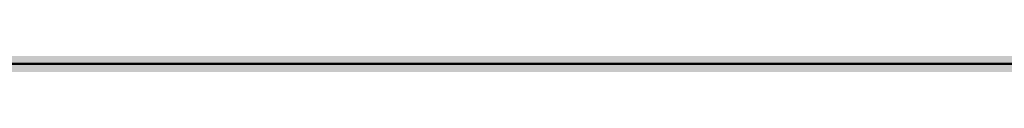
# Model space of a CAD drawing. Units: millimetres. Extents: x 0 to 2267, y 0 to 1823.
# Tile 113 of 256: x 1600.369 to 1605.705, y 1232.247 to 1232.247. Entities that reach past the tile are written whole.
import ezdxf

# ---------------------------------------------------------------- set-up
doc = ezdxf.new("R2010")
doc.units = ezdxf.units.MM
doc.header["$MEASUREMENT"] = 0
doc.layers.add('M-HATC', color=252, linetype='Continuous', lineweight=18)
doc.layers.add('M-OUTL', color=7, linetype='Continuous', lineweight=50)

msp = doc.modelspace()

# ---------------------------------------------------------------- hatches: boundary and pattern name
at = {"layer": 'M-HATC'}
h = msp.add_hatch(color=256, dxfattribs=at)
h.dxf.hatch_style = 1
h.paths.add_polyline_path([(2065.771, 1618.062, 0.236068), (2055.771, 1638.062), (1381.0868, 1638.062, 0.236068), (1371.0868, 1618.062), (1371.0868, 1603.062), (2055.771, 1603.062), (2065.771, 1603.062)])
h.paths.add_polyline_path([(2062.7718, 1550.2964), (2062.7718, 1560.2964), (1374.086, 1560.2964), (1374.086, 1550.2964), (1374.086, 1540.2964), (1384.086, 1540.2964), (1389.086, 1540.2964), (2062.7718, 1540.2964)])
h.paths.add_polyline_path([(1930.9289, 1282.7656), (1505.9289, 1282.7656), (1587.6276, 1235.5968, 0.131652), (1600.1276, 1232.2475), (1836.7302, 1232.2475, 0.131652), (1849.2302, 1235.5968)])
h.paths.add_polyline_path([(1930.9289, 1117.4171), (1905.9289, 1117.4171), (1505.9289, 1117.4171), (1505.9289, 1077.4171), (1930.9289, 1077.4171)])
h = msp.add_hatch(color=256, dxfattribs=at)
h.dxf.hatch_style = 1
h.paths.add_polyline_path([(2055.771, 1603.062), (1381.0868, 1603.062), (1381.0868, 1598.062), (2055.771, 1598.062)])
h.paths.add_polyline_path([(2055.771, 1598.062), (1381.0868, 1598.062), (1381.0868, 1593.062), (2055.771, 1593.062)])
h.paths.add_polyline_path([(2051.3074, 1536.7609), (1385.5504, 1536.7609), (1385.5504, 1526.7609), (1387.5504, 1526.7609), (1388.5366, 1525.0528), (1385.3319, 1521.2335), (1385.3319, 1521.2226), (2050.2542, 1522.7491), (2048.3212, 1525.0528), (2049.3074, 1526.7609), (2051.3074, 1526.7609)])
edge = h.paths.add_edge_path()
edge.add_arc((1847.5345, 1379.1492), 135, 222.603061, 222.890851, ccw=False)
edge.add_line((1748.1663, 1287.7656), (1683.0921, 1287.7656))
edge.add_arc((1583.7239, 1379.1492), 135, 317.109149, 317.396939, ccw=False)
edge.add_arc((1678.9686, 1290.6707), 5, 222.8909, 317.1091, ccw=False)
edge.add_arc((1774.2133, 1379.1492), 135, 222.603061, 222.890851, ccw=False)
edge.add_line((1674.8451, 1287.7656), (1609.7709, 1287.7656))
edge.add_arc((1510.4027, 1379.1492), 135, 317.109149, 317.396939, ccw=False)
edge.add_arc((1605.6474, 1290.6707), 5, 222.8909, 317.1091, ccw=False)
edge.add_arc((1700.8921, 1379.1492), 135, 222.603061, 222.890851, ccw=False)
edge.add_line((1601.5239, 1287.7656), (1536.4497, 1287.7656))
edge.add_arc((1437.0815, 1379.1492), 135, 317.109149, 317.396939, ccw=False)
edge.add_arc((1532.3262, 1290.6707), 5, 222.8909, 317.1091, ccw=False)
edge.add_arc((1627.5709, 1379.1492), 135, 222.603061, 222.890851, ccw=False)
edge.add_line((1528.2027, 1287.7656), (1505.9289, 1287.7656))
edge.add_spline(control_points=[(1505.9289, 1287.7656), (1504.2622, 1287.7656), (1504.2622, 1282.7656), (1505.9289, 1282.7656)], knot_values=[0, 0, 0, 0, 5, 5, 5, 5], degree=3, periodic=0)
edge.add_line((1505.9289, 1282.7656), (1930.9289, 1282.7656))
edge.add_spline(control_points=[(1930.9289, 1282.7656), (1932.5956, 1282.7656), (1932.5956, 1287.7656), (1930.9289, 1287.7656)], knot_values=[0, 0, 0, 0, 5, 5, 5, 5], degree=3, periodic=0)
edge.add_line((1930.9289, 1287.7656), (1903.0557, 1287.7656))
edge.add_arc((1803.6875, 1379.1492), 135, 317.109149, 317.396939, ccw=False)
edge.add_arc((1898.9322, 1290.6707), 5, 222.8909, 317.1091, ccw=False)
edge.add_arc((1994.1769, 1379.1492), 135, 222.603061, 222.890851, ccw=False)
edge.add_line((1894.8087, 1287.7656), (1829.7345, 1287.7656))
edge.add_arc((1730.3663, 1379.1492), 135, 317.109149, 317.396939, ccw=False)
edge.add_arc((1825.611, 1290.6707), 5, 222.8909, 317.1091, ccw=False)
edge.add_arc((1920.8557, 1379.1492), 135, 222.603061, 222.890851, ccw=False)
edge.add_line((1821.4875, 1287.7656), (1756.4133, 1287.7656))
edge.add_arc((1657.0451, 1379.1492), 135, 317.109149, 317.396939, ccw=False)
edge.add_arc((1752.2898, 1290.6707), 5, 222.8909, 317.1091, ccw=False)
edge = h.paths.add_edge_path()
edge.add_spline(control_points=[(1843.4289, 1227.2475), (1845.0956, 1227.2475), (1845.0956, 1232.2475), (1843.4289, 1232.2475)], knot_values=[0, 0, 0, 0, 5, 5, 5, 5], degree=3, periodic=0)
edge.add_line((1843.4289, 1232.2475), (1593.4289, 1232.2475))
edge.add_spline(control_points=[(1593.4289, 1232.2475), (1591.7622, 1232.2475), (1591.7622, 1227.2475), (1593.4289, 1227.2475)], knot_values=[0, 0, 0, 0, 5, 5, 5, 5], degree=3, periodic=0)
edge.add_line((1593.4289, 1227.2475), (1843.4289, 1227.2475))
h.paths.add_polyline_path([(1905.9289, 1127.4171), (1530.9289, 1127.4171, 0.414214), (1520.9289, 1117.4171), (1530.9289, 1117.4171), (1915.9289, 1117.4171, 0.414214)])
edge = h.paths.add_edge_path()
edge.add_arc((1397.0858, 1498.4078), 12.7299, 90.78215, 190.87871, ccw=False)
edge.add_line((1396.912, 1511.1365), (1428.0097, 1511.3488))
edge.add_line((1428.0097, 1511.3488), (1433.0097, 1511.3488))
edge.add_line((1433.0097, 1511.3488), (1434.439, 1511.3488))
edge.add_arc((1419.474, 1498.0804), 20, 41.561, 74.08211)
edge.add_line((1424.9592, 1517.3135), (1399.9351, 1517.2561))
edge.add_spline(control_points=[(1399.9307, 1517.2561), (1399.884, 1517.2131), (1399.8328, 1517.1689), (1399.7774, 1517.1236)], knot_values=[11.567499, 11.567499, 11.567499, 11.567499, 11.814249, 11.814249, 11.814249, 11.814249], degree=3, periodic=0)
edge.add_spline(control_points=[(1399.6328, 1517.0099), (1399.5831, 1516.9721), (1399.5307, 1516.9338), (1399.4759, 1516.8947)], knot_values=[11.167718, 11.167718, 11.167718, 11.167718, 11.365188, 11.365188, 11.365188, 11.365188], degree=3, periodic=0)
edge.add_spline(control_points=[(1399.3398, 1516.8001), (1399.1514, 1516.6719), (1398.9384, 1516.5377), (1398.704, 1516.3994)], knot_values=[10.376405, 10.376405, 10.376405, 10.376405, 11.00994, 11.00994, 11.00994, 11.00994], degree=3, periodic=0)
edge.add_spline(control_points=[(1398.6572, 1516.3719), (1398.5789, 1516.326), (1398.4983, 1516.2797), (1398.4155, 1516.2331)], knot_values=[10.125175, 10.125175, 10.125175, 10.125175, 10.334406, 10.334406, 10.334406, 10.334406], degree=3, periodic=0)
edge.add_spline(control_points=[(1398.2642, 1516.1487), (1398.196, 1516.1111), (1398.1263, 1516.0732), (1398.0555, 1516.0351)], knot_values=[9.832246, 9.832246, 9.832246, 9.832246, 9.999658, 9.999658, 9.999658, 9.999658], degree=3, periodic=0)
edge.add_spline(control_points=[(1397.9987, 1516.0048), (1397.7312, 1515.8621), (1397.446, 1515.7171), (1397.1466, 1515.5714)], knot_values=[9.161808, 9.161808, 9.161808, 9.161808, 9.787769, 9.787769, 9.787769, 9.787769], degree=3, periodic=0)
edge.add_spline(control_points=[(1397.1466, 1515.5714), (1396.8418, 1515.423), (1396.5222, 1515.274), (1396.1914, 1515.1262)], knot_values=[8.524455, 8.524455, 8.524455, 8.524455, 9.161808, 9.161808, 9.161808, 9.161808], degree=3, periodic=0)
edge.add_spline(control_points=[(1396.0777, 1515.0756), (1395.9854, 1515.0348), (1395.8922, 1514.994), (1395.7983, 1514.9534)], knot_values=[8.275193, 8.275193, 8.275193, 8.275193, 8.451726, 8.451726, 8.451726, 8.451726], degree=3, periodic=0)
edge.add_spline(control_points=[(1395.6018, 1514.8691), (1395.4997, 1514.8257), (1395.3968, 1514.7824), (1395.2932, 1514.7394)], knot_values=[7.962917, 7.962917, 7.962917, 7.962917, 8.152764, 8.152764, 8.152764, 8.152764], degree=3, periodic=0)
edge.add_spline(control_points=[(1395.2116, 1514.7057), (1394.8278, 1514.5475), (1394.4345, 1514.3929), (1394.0364, 1514.2442)], knot_values=[7.21254, 7.21254, 7.21254, 7.21254, 7.913148, 7.913148, 7.913148, 7.913148], degree=3, periodic=0)
edge.add_spline(control_points=[(1394.0364, 1514.2442), (1393.7076, 1514.1214), (1393.3754, 1514.0027), (1393.0427, 1513.8895)], knot_values=[6.633733, 6.633733, 6.633733, 6.633733, 7.21254, 7.21254, 7.21254, 7.21254], degree=3, periodic=0)
edge.add_spline(control_points=[(1392.8214, 1513.815), (1392.7198, 1513.7812), (1392.6181, 1513.7479), (1392.5166, 1513.7152)], knot_values=[6.328796, 6.328796, 6.328796, 6.328796, 6.505493, 6.505493, 6.505493, 6.505493], degree=3, periodic=0)
edge.add_spline(control_points=[(1392.5166, 1513.7152), (1392.3187, 1513.6515), (1392.1212, 1513.59), (1391.9244, 1513.531)], knot_values=[5.984605, 5.984605, 5.984605, 5.984605, 6.328796, 6.328796, 6.328796, 6.328796], degree=3, periodic=0)
edge.add_spline(control_points=[(1391.7915, 1513.4915), (1391.3122, 1513.3501), (1390.8384, 1513.2239), (1390.3784, 1513.1171)], knot_values=[5.066697, 5.066697, 5.066697, 5.066697, 5.907055, 5.907055, 5.907055, 5.907055], degree=3, periodic=0)
edge.add_spline(control_points=[(1390.3784, 1513.1171), (1390.1797, 1513.071), (1389.9836, 1513.0284), (1389.7907, 1512.9899)], knot_values=[4.70367, 4.70367, 4.70367, 4.70367, 5.066695, 5.066695, 5.066695, 5.066695], degree=3, periodic=0)
edge.add_spline(control_points=[(1389.422, 1512.9204), (1389.2459, 1512.8892), (1389.0729, 1512.8617), (1388.9036, 1512.8381)], knot_values=[4.130571, 4.130571, 4.130571, 4.130571, 4.469816, 4.469816, 4.469816, 4.469816], degree=3, periodic=0)
edge.add_spline(control_points=[(1388.9036, 1512.8381), (1388.591, 1512.7946), (1388.2911, 1512.7644), (1388.0071, 1512.7494)], knot_values=[3.504031, 3.504031, 3.504031, 3.504031, 4.130571, 4.130571, 4.130571, 4.130571], degree=3, periodic=0)
edge.add_spline(control_points=[(1387.9356, 1512.7459), (1387.8538, 1512.7423), (1387.7733, 1512.74), (1387.6944, 1512.739)], knot_values=[3.268866, 3.268866, 3.268866, 3.268866, 3.451164, 3.451164, 3.451164, 3.451164], degree=3, periodic=0)
edge.add_spline(control_points=[(1387.3351, 1512.7443), (1387.2076, 1512.7499), (1387.0847, 1512.7597), (1386.967, 1512.7739)], knot_values=[2.670686, 2.670686, 2.670686, 2.670686, 2.984, 2.984, 2.984, 2.984], degree=3, periodic=0)
edge.add_spline(control_points=[(1386.8327, 1512.7922), (1386.8209, 1512.7941), (1386.8092, 1512.7959), (1386.7975, 1512.7979)], knot_values=[2.516981, 2.516981, 2.516981, 2.516981, 2.549528, 2.549528, 2.549528, 2.549528], degree=3, periodic=0)
edge.add_spline(control_points=[(1386.4526, 1512.8735), (1386.4257, 1512.881), (1386.3993, 1512.889), (1386.3733, 1512.8972)], knot_values=[2.095869, 2.095869, 2.095869, 2.095869, 2.17941, 2.17941, 2.17941, 2.17941], degree=3, periodic=0)
edge.add_spline(control_points=[(1386.0691, 1513.0189), (1386.0634, 1513.0217), (1386.0577, 1513.0246), (1386.052, 1513.0275)], knot_values=[1.72453, 1.72453, 1.72453, 1.72453, 1.745933, 1.745933, 1.745933, 1.745933], degree=3, periodic=0)
edge.add_arc((1399.474, 1498.0804), 20, 131.82432, 180)
edge.add_arc((1630.3336, 1505.5484), 250.9708, 181.705176, 236.427975)
edge.add_arc((1605.3399, 1483.3044), 218.7822, 238.660829, 243.34961)
edge.add_arc((1647.0911, 1510.3592), 262.8986, 183.129836, 237.853442, ccw=False)
h.paths.add_polyline_path([(1406.5369, 1391.9644, 0.149382), (1491.5506, 1296.4418, -0.129517)], flags=17)
edge = h.paths.add_edge_path()
edge.add_arc((2037.3838, 1498.0804), 20, 0, 48.26587)
edge.add_spline(control_points=[(2050.6973, 1513.0052), (2050.6512, 1512.9847), (2050.6034, 1512.9655), (2050.5539, 1512.9477)], knot_values=[1.835652, 1.835652, 1.835652, 1.835652, 2.000781, 2.000781, 2.000781, 2.000781], degree=3, periodic=0)
edge.add_spline(control_points=[(2050.4616, 1512.9166), (2050.479, 1512.9221), (2050.4963, 1512.9277), (2050.5133, 1512.9335)], knot_values=[2.045477, 2.045477, 2.045477, 2.045477, 2.101389, 2.101389, 2.101389, 2.101389], degree=3, periodic=0)
edge.add_spline(control_points=[(2050.129, 1512.8342), (2050.1984, 1512.8473), (2050.2657, 1512.8623), (2050.3308, 1512.8792)], knot_values=[2.237629, 2.237629, 2.237629, 2.237629, 2.435841, 2.435841, 2.435841, 2.435841], degree=3, periodic=0)
edge.add_spline(control_points=[(2050.0946, 1512.8278), (2050.1061, 1512.8299), (2050.1176, 1512.832), (2050.129, 1512.8342)], knot_values=[2.435841, 2.435841, 2.435841, 2.435841, 2.468321, 2.468321, 2.468321, 2.468321], degree=3, periodic=0)
edge.add_spline(control_points=[(2049.7843, 1512.7851), (2049.8552, 1512.7922), (2049.9243, 1512.8008), (2049.9917, 1512.8109)], knot_values=[2.563852, 2.563852, 2.563852, 2.563852, 2.748541, 2.748541, 2.748541, 2.748541], degree=3, periodic=0)
edge.add_spline(control_points=[(2049.4052, 1512.7617), (2049.5364, 1512.7653), (2049.6629, 1512.773), (2049.7843, 1512.7851)], knot_values=[2.748541, 2.748541, 2.748541, 2.748541, 3.064882, 3.064882, 3.064882, 3.064882], degree=3, periodic=0)
edge.add_spline(control_points=[(2049.1698, 1512.7597), (2049.2336, 1512.7591), (2049.2965, 1512.7594), (2049.3584, 1512.7606)], knot_values=[3.102309, 3.102309, 3.102309, 3.102309, 3.2503, 3.2503, 3.2503, 3.2503], degree=3, periodic=0)
edge.add_spline(control_points=[(2048.8573, 1512.7691), (2048.9638, 1512.7638), (2049.068, 1512.7606), (2049.1698, 1512.7597)], knot_values=[3.2503, 3.2503, 3.2503, 3.2503, 3.486069, 3.486069, 3.486069, 3.486069], degree=3, periodic=0)
edge.add_spline(control_points=[(2048.6924, 1512.7789), (2048.3729, 1512.8009), (2048.0345, 1512.8411), (2047.6817, 1512.897)], knot_values=[3.606429, 3.606429, 3.606429, 3.606429, 4.2989, 4.2989, 4.2989, 4.2989], degree=3, periodic=0)
edge.add_spline(control_points=[(2047.6817, 1512.897), (2047.5458, 1512.9185), (2047.4077, 1512.9424), (2047.2678, 1512.9685)], knot_values=[4.2989, 4.2989, 4.2989, 4.2989, 4.565769, 4.565769, 4.565769, 4.565769], degree=3, periodic=0)
edge.add_spline(control_points=[(2047.2678, 1512.9685), (2047.1449, 1512.9914), (2047.0207, 1513.016), (2046.8951, 1513.0422)], knot_values=[4.565769, 4.565769, 4.565769, 4.565769, 4.799971, 4.799971, 4.799971, 4.799971], degree=3, periodic=0)
edge.add_spline(control_points=[(2046.8951, 1513.0422), (2046.5286, 1513.1188), (2046.1513, 1513.209), (2045.7676, 1513.3107)], knot_values=[4.799971, 4.799971, 4.799971, 4.799971, 5.483718, 5.483718, 5.483718, 5.483718], degree=3, periodic=0)
edge.add_spline(control_points=[(2045.7676, 1513.3107), (2045.3724, 1513.4154), (2044.9704, 1513.5322), (2044.5662, 1513.6588)], knot_values=[5.483718, 5.483718, 5.483718, 5.483718, 6.187866, 6.187866, 6.187866, 6.187866], degree=3, periodic=0)
edge.add_spline(control_points=[(2044.5662, 1513.6588), (2044.4149, 1513.7061), (2044.2633, 1513.7549), (2044.1116, 1513.8048)], knot_values=[6.187866, 6.187866, 6.187866, 6.187866, 6.451551, 6.451551, 6.451551, 6.451551], degree=3, periodic=0)
edge.add_spline(control_points=[(2044.1116, 1513.8048), (2043.9967, 1513.8427), (2043.8817, 1513.8813), (2043.7668, 1513.9205)], knot_values=[6.451551, 6.451551, 6.451551, 6.451551, 6.651434, 6.651434, 6.651434, 6.651434], degree=3, periodic=0)
edge.add_spline(control_points=[(2043.7668, 1513.9205), (2043.3716, 1514.0554), (2042.9774, 1514.1979), (2042.5886, 1514.3458)], knot_values=[6.651434, 6.651434, 6.651434, 6.651434, 7.338879, 7.338879, 7.338879, 7.338879], degree=3, periodic=0)
edge.add_spline(control_points=[(2042.5886, 1514.3458), (2042.1643, 1514.5071), (2041.7465, 1514.6749), (2041.3409, 1514.846)], knot_values=[7.338879, 7.338879, 7.338879, 7.338879, 8.089209, 8.089209, 8.089209, 8.089209], degree=3, periodic=0)
edge.add_spline(control_points=[(2041.3409, 1514.846), (2041.1028, 1514.9465), (2040.869, 1515.0481), (2040.6405, 1515.1502)], knot_values=[8.089209, 8.089209, 8.089209, 8.089209, 8.529587, 8.529587, 8.529587, 8.529587], degree=3, periodic=0)
edge.add_spline(control_points=[(2040.51, 1515.2089), (2040.0824, 1515.4022), (2039.6747, 1515.5971), (2039.295, 1515.7894)], knot_values=[8.613818, 8.613818, 8.613818, 8.613818, 9.44571, 9.44571, 9.44571, 9.44571], degree=3, periodic=0)
edge.add_spline(control_points=[(2039.295, 1515.7894), (2039.0618, 1515.9075), (2038.8391, 1516.0246), (2038.6288, 1516.1398)], knot_values=[9.44571, 9.44571, 9.44571, 9.44571, 9.956404, 9.956404, 9.956404, 9.956404], degree=3, periodic=0)
edge.add_spline(control_points=[(2038.6288, 1516.1398), (2038.5187, 1516.2001), (2038.4121, 1516.2598), (2038.309, 1516.3189)], knot_values=[9.956404, 9.956404, 9.956404, 9.956404, 10.223542, 10.223542, 10.223542, 10.223542], degree=3, periodic=0)
edge.add_spline(control_points=[(2038.309, 1516.3189), (2038.2138, 1516.3735), (2038.1216, 1516.4276), (2038.0328, 1516.481)], knot_values=[10.223542, 10.223542, 10.223542, 10.223542, 10.47051, 10.47051, 10.47051, 10.47051], degree=3, periodic=0)
edge.add_spline(control_points=[(2038.0328, 1516.481), (2037.7855, 1516.6296), (2037.5639, 1516.773), (2037.3722, 1516.909)], knot_values=[10.47051, 10.47051, 10.47051, 10.47051, 11.15767, 11.15767, 11.15767, 11.15767], degree=3, periodic=0)
edge.add_spline(control_points=[(2037.3722, 1516.909), (2037.2789, 1516.9752), (2037.1927, 1517.0396), (2037.1142, 1517.102)], knot_values=[11.15767, 11.15767, 11.15767, 11.15767, 11.49227, 11.49227, 11.49227, 11.49227], degree=3, periodic=0)
edge.add_spline(control_points=[(2036.8564, 1517.3259), (2036.9148, 1517.2692), (2036.9814, 1517.2103), (2037.0557, 1517.1492)], knot_values=[11.577341, 11.577341, 11.577341, 11.577341, 11.91035, 11.91035, 11.91035, 11.91035], degree=3, periodic=0)
edge.add_spline(control_points=[(2036.8074, 1517.3748), (2036.823, 1517.3587), (2036.8393, 1517.3424), (2036.8564, 1517.3259)], knot_values=[11.91035, 11.91035, 11.91035, 11.91035, 12.007402, 12.007402, 12.007402, 12.007402], degree=3, periodic=0)
edge.add_spline(control_points=[(2036.7017, 1517.494), (2036.7104, 1517.483), (2036.7196, 1517.4719), (2036.7291, 1517.4606)], knot_values=[12.184155, 12.184155, 12.184155, 12.184155, 12.255409, 12.255409, 12.255409, 12.255409], degree=3, periodic=0)
edge.add_spline(control_points=[(2036.6159, 1517.6205), (2036.62, 1517.613), (2036.6243, 1517.6055), (2036.6289, 1517.5979)], knot_values=[12.487913, 12.487913, 12.487913, 12.487913, 12.541035, 12.541035, 12.541035, 12.541035], degree=3, periodic=0)
edge.add_spline(control_points=[(2036.5635, 1517.786), (2036.5637, 1517.7794), (2036.5642, 1517.7726), (2036.565, 1517.7658)], knot_values=[12.911761, 12.911761, 12.911761, 12.911761, 12.968286, 12.968286, 12.968286, 12.968286], degree=3, periodic=0)
edge.add_spline(control_points=[(2036.6166, 1517.9304), (2036.6125, 1517.9259), (2036.6086, 1517.9212), (2036.6049, 1517.9165)], knot_values=[13.382527, 13.382527, 13.382527, 13.382527, 13.433791, 13.433791, 13.433791, 13.433791], degree=3, periodic=0)
edge.add_spline(control_points=[(2036.749, 1518.017), (2036.7361, 1518.0116), (2036.7239, 1518.006), (2036.7124, 1518.0002)], knot_values=[13.726299, 13.726299, 13.726299, 13.726299, 13.809928, 13.809928, 13.809928, 13.809928], degree=3, periodic=0)
edge.add_spline(control_points=[(2036.8604, 1518.0528), (2036.8386, 1518.0474), (2036.8181, 1518.0416), (2036.7988, 1518.0353)], knot_values=[13.910887, 13.910887, 13.910887, 13.910887, 14.02153, 14.02153, 14.02153, 14.02153], degree=3, periodic=0)
edge.add_line((2036.9639, 1518.0804), (2032.3838, 1518.0804))
edge.add_line((2032.3838, 1518.0804), (2027.3838, 1518.0804))
edge.add_line((2027.3838, 1518.0804), (2022.3838, 1518.0804))
edge.add_line((2022.3838, 1518.0804), (2017.3838, 1518.0804))
edge.add_arc((2017.3838, 1498.0804), 20, 90, 138.439)
edge.add_line((2002.4188, 1511.3488), (2003.8481, 1511.3488))
edge.add_line((2003.8481, 1511.3488), (2008.8481, 1511.3488))
edge.add_line((2008.8481, 1511.3488), (2039.772, 1511.1377))
edge.add_arc((2039.772, 1498.4078), 12.7299, -10.87871, 90, ccw=False)
edge.add_arc((1789.7668, 1510.3592), 262.8986, 302.146558, 356.870164, ccw=False)
edge.add_arc((1831.5179, 1483.3044), 218.7822, 296.65039, 301.339171)
edge.add_arc((1806.5242, 1505.5484), 250.9708, 303.572025, 358.294824)
h.paths.add_polyline_path([(2030.321, 1391.9644, -0.129517), (1945.3072, 1296.4418, 0.149382)], flags=17)
edge = h.paths.add_edge_path()
edge.add_spline(control_points=[(2037.2464, 1518.0821), (2037.2898, 1518.081), (2037.3355, 1518.0804), (2037.3838, 1518.0804)], knot_values=[0.000012, 0.000012, 0.000012, 0.000012, 0.144754, 0.144754, 0.144754, 0.144754], degree=3, periodic=0)
edge.add_line((2037.3357, 1518.0804), (2037.0096, 1518.0804))
edge.add_spline(control_points=[(2037.0096, 1518.0804), (2036.9822, 1518.0768), (2036.956, 1518.0727), (2036.9312, 1518.0681)], knot_values=[14.13465, 14.13465, 14.13465, 14.13465, 14.247197, 14.247197, 14.247197, 14.247197], degree=3, periodic=0)
edge.add_spline(control_points=[(2036.9312, 1518.0681), (2036.9276, 1518.0674), (2036.9241, 1518.0667), (2036.9205, 1518.0661)], knot_values=[14.118315, 14.118315, 14.118315, 14.118315, 14.13465, 14.13465, 14.13465, 14.13465], degree=3, periodic=0)
edge.add_spline(control_points=[(2036.9205, 1518.0661), (2036.9118, 1518.0644), (2036.9032, 1518.0626), (2036.8948, 1518.0608)], knot_values=[14.078086, 14.078086, 14.078086, 14.078086, 14.118315, 14.118315, 14.118315, 14.118315], degree=3, periodic=0)
edge.add_spline(control_points=[(2036.8948, 1518.0608), (2036.883, 1518.0583), (2036.8716, 1518.0556), (2036.8604, 1518.0528)], knot_values=[14.02153, 14.02153, 14.02153, 14.02153, 14.078086, 14.078086, 14.078086, 14.078086], degree=3, periodic=0)
edge.add_spline(control_points=[(2036.8604, 1518.0528), (2036.8386, 1518.0474), (2036.8181, 1518.0416), (2036.7988, 1518.0353)], knot_values=[13.910887, 13.910887, 13.910887, 13.910887, 14.02153, 14.02153, 14.02153, 14.02153], degree=3, periodic=0)
edge.add_spline(control_points=[(2036.7988, 1518.0353), (2036.7981, 1518.035), (2036.7974, 1518.0348), (2036.7967, 1518.0346)], knot_values=[13.906906, 13.906906, 13.906906, 13.906906, 13.910887, 13.910887, 13.910887, 13.910887], degree=3, periodic=0)
edge.add_spline(control_points=[(2036.7967, 1518.0346), (2036.7882, 1518.0318), (2036.7799, 1518.0289), (2036.7719, 1518.0259)], knot_values=[13.857826, 13.857826, 13.857826, 13.857826, 13.906906, 13.906906, 13.906906, 13.906906], degree=3, periodic=0)
edge.add_spline(control_points=[(2036.7719, 1518.0259), (2036.764, 1518.023), (2036.7564, 1518.02), (2036.749, 1518.017)], knot_values=[13.809928, 13.809928, 13.809928, 13.809928, 13.857826, 13.857826, 13.857826, 13.857826], degree=3, periodic=0)
edge.add_spline(control_points=[(2036.749, 1518.017), (2036.7361, 1518.0116), (2036.7239, 1518.006), (2036.7124, 1518.0002)], knot_values=[13.726299, 13.726299, 13.726299, 13.726299, 13.809928, 13.809928, 13.809928, 13.809928], degree=3, periodic=0)
edge.add_spline(control_points=[(2036.7124, 1518.0002), (2036.7121, 1518), (2036.7118, 1517.9999), (2036.7115, 1517.9997)], knot_values=[13.723993, 13.723993, 13.723993, 13.723993, 13.726299, 13.726299, 13.726299, 13.726299], degree=3, periodic=0)
edge.add_spline(control_points=[(2036.7115, 1517.9997), (2036.7063, 1517.9971), (2036.7013, 1517.9944), (2036.6965, 1517.9917)], knot_values=[13.686536, 13.686536, 13.686536, 13.686536, 13.723993, 13.723993, 13.723993, 13.723993], degree=3, periodic=0)
edge.add_spline(control_points=[(2036.6965, 1517.9917), (2036.6919, 1517.9891), (2036.6874, 1517.9865), (2036.6831, 1517.9839)], knot_values=[13.651251, 13.651251, 13.651251, 13.651251, 13.686536, 13.686536, 13.686536, 13.686536], degree=3, periodic=0)
edge.add_spline(control_points=[(2036.6831, 1517.9839), (2036.6764, 1517.9798), (2036.67, 1517.9757), (2036.6639, 1517.9714)], knot_values=[13.596804, 13.596804, 13.596804, 13.596804, 13.651251, 13.651251, 13.651251, 13.651251], degree=3, periodic=0)
edge.add_spline(control_points=[(2036.6639, 1517.9714), (2036.6636, 1517.9712), (2036.6633, 1517.9709), (2036.6629, 1517.9707)], knot_values=[13.593956, 13.593956, 13.593956, 13.593956, 13.596804, 13.596804, 13.596804, 13.596804], degree=3, periodic=0)
edge.add_spline(control_points=[(2036.6629, 1517.9707), (2036.6603, 1517.9689), (2036.6577, 1517.967), (2036.6552, 1517.9651)], knot_values=[13.570322, 13.570322, 13.570322, 13.570322, 13.593956, 13.593956, 13.593956, 13.593956], degree=3, periodic=0)
edge.add_spline(control_points=[(2036.6552, 1517.9651), (2036.6525, 1517.9631), (2036.6499, 1517.9611), (2036.6474, 1517.9591)], knot_values=[13.545477, 13.545477, 13.545477, 13.545477, 13.570322, 13.570322, 13.570322, 13.570322], degree=3, periodic=0)
edge.add_spline(control_points=[(2036.6474, 1517.9591), (2036.6472, 1517.9589), (2036.6471, 1517.9588), (2036.6469, 1517.9587)], knot_values=[13.543931, 13.543931, 13.543931, 13.543931, 13.545477, 13.545477, 13.545477, 13.545477], degree=3, periodic=0)
edge.add_spline(control_points=[(2036.6469, 1517.9587), (2036.6412, 1517.9541), (2036.6358, 1517.9494), (2036.6307, 1517.9447)], knot_values=[13.488237, 13.488237, 13.488237, 13.488237, 13.543931, 13.543931, 13.543931, 13.543931], degree=3, periodic=0)
edge.add_spline(control_points=[(2036.6307, 1517.9447), (2036.6282, 1517.9423), (2036.6257, 1517.9399), (2036.6233, 1517.9374)], knot_values=[13.460307, 13.460307, 13.460307, 13.460307, 13.488237, 13.488237, 13.488237, 13.488237], degree=3, periodic=0)
edge.add_spline(control_points=[(2036.6233, 1517.9374), (2036.6215, 1517.9356), (2036.6198, 1517.9338), (2036.6181, 1517.932)], knot_values=[13.439712, 13.439712, 13.439712, 13.439712, 13.460307, 13.460307, 13.460307, 13.460307], degree=3, periodic=0)
edge.add_spline(control_points=[(2036.6181, 1517.932), (2036.6176, 1517.9315), (2036.6171, 1517.9309), (2036.6166, 1517.9304)], knot_values=[13.433791, 13.433791, 13.433791, 13.433791, 13.439712, 13.439712, 13.439712, 13.439712], degree=3, periodic=0)
edge.add_spline(control_points=[(2036.6166, 1517.9304), (2036.6125, 1517.9259), (2036.6086, 1517.9212), (2036.6049, 1517.9165)], knot_values=[13.382527, 13.382527, 13.382527, 13.382527, 13.433791, 13.433791, 13.433791, 13.433791], degree=3, periodic=0)
edge.add_spline(control_points=[(2036.6049, 1517.9165), (2036.6026, 1517.9135), (2036.6004, 1517.9104), (2036.5982, 1517.9074)], knot_values=[13.350017, 13.350017, 13.350017, 13.350017, 13.382527, 13.382527, 13.382527, 13.382527], degree=3, periodic=0)
edge.add_spline(control_points=[(2036.5982, 1517.9074), (2036.5972, 1517.9059), (2036.5962, 1517.9043), (2036.5952, 1517.9028)], knot_values=[13.333922, 13.333922, 13.333922, 13.333922, 13.350017, 13.350017, 13.350017, 13.350017], degree=3, periodic=0)
edge.add_spline(control_points=[(2036.5952, 1517.9028), (2036.5945, 1517.9018), (2036.5939, 1517.9009), (2036.5933, 1517.8999)], knot_values=[13.323828, 13.323828, 13.323828, 13.323828, 13.333922, 13.333922, 13.333922, 13.333922], degree=3, periodic=0)
edge.add_spline(control_points=[(2036.5933, 1517.8999), (2036.5905, 1517.8955), (2036.5879, 1517.8909), (2036.5855, 1517.8864)], knot_values=[13.277545, 13.277545, 13.277545, 13.277545, 13.323828, 13.323828, 13.323828, 13.323828], degree=3, periodic=0)
edge.add_spline(control_points=[(2036.5855, 1517.8864), (2036.5836, 1517.8827), (2036.5817, 1517.8789), (2036.5801, 1517.8751)], knot_values=[13.240119, 13.240119, 13.240119, 13.240119, 13.277545, 13.277545, 13.277545, 13.277545], degree=3, periodic=0)
edge.add_spline(control_points=[(2036.5801, 1517.8751), (2036.5795, 1517.8739), (2036.579, 1517.8727), (2036.5785, 1517.8715)], knot_values=[13.228211, 13.228211, 13.228211, 13.228211, 13.240119, 13.240119, 13.240119, 13.240119], degree=3, periodic=0)
edge.add_spline(control_points=[(2036.5785, 1517.8715), (2036.578, 1517.8702), (2036.5774, 1517.869), (2036.5769, 1517.8677)], knot_values=[13.215717, 13.215717, 13.215717, 13.215717, 13.228211, 13.228211, 13.228211, 13.228211], degree=3, periodic=0)
edge.add_spline(control_points=[(2036.5769, 1517.8677), (2036.5755, 1517.864), (2036.5741, 1517.8603), (2036.5729, 1517.8565)], knot_values=[13.179847, 13.179847, 13.179847, 13.179847, 13.215717, 13.215717, 13.215717, 13.215717], degree=3, periodic=0)
edge.add_spline(control_points=[(2036.5729, 1517.8565), (2036.5713, 1517.8515), (2036.5699, 1517.8464), (2036.5687, 1517.8413)], knot_values=[13.132017, 13.132017, 13.132017, 13.132017, 13.179847, 13.179847, 13.179847, 13.179847], degree=3, periodic=0)
edge.add_spline(control_points=[(2036.5687, 1517.8413), (2036.5684, 1517.8402), (2036.5682, 1517.8392), (2036.568, 1517.8382)], knot_values=[13.122482, 13.122482, 13.122482, 13.122482, 13.132017, 13.132017, 13.132017, 13.132017], degree=3, periodic=0)
edge.add_spline(control_points=[(2036.568, 1517.8382), (2036.5676, 1517.8363), (2036.5672, 1517.8345), (2036.5669, 1517.8327)], knot_values=[13.105592, 13.105592, 13.105592, 13.105592, 13.122482, 13.122482, 13.122482, 13.122482], degree=3, periodic=0)
edge.add_spline(control_points=[(2036.5669, 1517.8327), (2036.5662, 1517.8292), (2036.5657, 1517.8257), (2036.5652, 1517.8222)], knot_values=[13.074063, 13.074063, 13.074063, 13.074063, 13.105592, 13.105592, 13.105592, 13.105592], degree=3, periodic=0)
edge.add_spline(control_points=[(2036.5652, 1517.8222), (2036.5652, 1517.8222), (2036.5652, 1517.8222), (2036.5652, 1517.8222)], knot_values=[13.074043, 13.074043, 13.074043, 13.074043, 13.074063, 13.074063, 13.074063, 13.074063], degree=3, periodic=0)
edge.add_spline(control_points=[(2036.5652, 1517.8222), (2036.5644, 1517.8164), (2036.5639, 1517.8106), (2036.5636, 1517.8046)], knot_values=[13.021884, 13.021884, 13.021884, 13.021884, 13.074043, 13.074043, 13.074043, 13.074043], degree=3, periodic=0)
edge.add_spline(control_points=[(2036.5636, 1517.8046), (2036.5636, 1517.804), (2036.5636, 1517.8034), (2036.5635, 1517.8028)], knot_values=[13.01674, 13.01674, 13.01674, 13.01674, 13.021884, 13.021884, 13.021884, 13.021884], degree=3, periodic=0)
edge.add_spline(control_points=[(2036.5635, 1517.8028), (2036.5634, 1517.8005), (2036.5634, 1517.7982), (2036.5634, 1517.7958)], knot_values=[12.996438, 12.996438, 12.996438, 12.996438, 13.01674, 13.01674, 13.01674, 13.01674], degree=3, periodic=0)
edge.add_spline(control_points=[(2036.5634, 1517.7958), (2036.5633, 1517.7926), (2036.5634, 1517.7893), (2036.5635, 1517.786)], knot_values=[12.968286, 12.968286, 12.968286, 12.968286, 12.996438, 12.996438, 12.996438, 12.996438], degree=3, periodic=0)
edge.add_spline(control_points=[(2036.5635, 1517.786), (2036.5637, 1517.7794), (2036.5642, 1517.7726), (2036.565, 1517.7658)], knot_values=[12.911761, 12.911761, 12.911761, 12.911761, 12.968286, 12.968286, 12.968286, 12.968286], degree=3, periodic=0)
edge.add_spline(control_points=[(2036.565, 1517.7658), (2036.565, 1517.7657), (2036.565, 1517.7656), (2036.565, 1517.7656)], knot_values=[12.911017, 12.911017, 12.911017, 12.911017, 12.911761, 12.911761, 12.911761, 12.911761], degree=3, periodic=0)
edge.add_spline(control_points=[(2036.565, 1517.7656), (2036.5654, 1517.7625), (2036.5658, 1517.7593), (2036.5663, 1517.7562)], knot_values=[12.88528, 12.88528, 12.88528, 12.88528, 12.911017, 12.911017, 12.911017, 12.911017], degree=3, periodic=0)
edge.add_spline(control_points=[(2036.5663, 1517.7562), (2036.5667, 1517.7534), (2036.5672, 1517.7506), (2036.5677, 1517.7478)], knot_values=[12.862519, 12.862519, 12.862519, 12.862519, 12.88528, 12.88528, 12.88528, 12.88528], degree=3, periodic=0)
edge.add_spline(control_points=[(2036.5677, 1517.7478), (2036.5678, 1517.7474), (2036.5679, 1517.7469), (2036.568, 1517.7465)], knot_values=[12.858885, 12.858885, 12.858885, 12.858885, 12.862519, 12.862519, 12.862519, 12.862519], degree=3, periodic=0)
edge.add_spline(control_points=[(2036.568, 1517.7465), (2036.5692, 1517.7399), (2036.5707, 1517.7332), (2036.5724, 1517.7264)], knot_values=[12.8053, 12.8053, 12.8053, 12.8053, 12.858885, 12.858885, 12.858885, 12.858885], degree=3, periodic=0)
edge.add_spline(control_points=[(2036.5724, 1517.7264), (2036.5734, 1517.7226), (2036.5745, 1517.7187), (2036.5756, 1517.7149)], knot_values=[12.775176, 12.775176, 12.775176, 12.775176, 12.8053, 12.8053, 12.8053, 12.8053], degree=3, periodic=0)
edge.add_spline(control_points=[(2036.5756, 1517.7149), (2036.5763, 1517.7125), (2036.577, 1517.7102), (2036.5778, 1517.7078)], knot_values=[12.756759, 12.756759, 12.756759, 12.756759, 12.775176, 12.775176, 12.775176, 12.775176], degree=3, periodic=0)
edge.add_spline(control_points=[(2036.5778, 1517.7078), (2036.5781, 1517.7067), (2036.5784, 1517.7057), (2036.5787, 1517.7047)], knot_values=[12.748742, 12.748742, 12.748742, 12.748742, 12.756759, 12.756759, 12.756759, 12.756759], degree=3, periodic=0)
edge.add_spline(control_points=[(2036.5787, 1517.7047), (2036.5808, 1517.6983), (2036.5831, 1517.6919), (2036.5856, 1517.6854)], knot_values=[12.69959, 12.69959, 12.69959, 12.69959, 12.748742, 12.748742, 12.748742, 12.748742], degree=3, periodic=0)
edge.add_spline(control_points=[(2036.5856, 1517.6854), (2036.5876, 1517.68), (2036.5898, 1517.6746), (2036.5921, 1517.6692)], knot_values=[12.659038, 12.659038, 12.659038, 12.659038, 12.69959, 12.69959, 12.69959, 12.69959], degree=3, periodic=0)
edge.add_spline(control_points=[(2036.5921, 1517.6692), (2036.594, 1517.6648), (2036.5959, 1517.6605), (2036.5979, 1517.6561)], knot_values=[12.626806, 12.626806, 12.626806, 12.626806, 12.659038, 12.659038, 12.659038, 12.659038], degree=3, periodic=0)
edge.add_spline(control_points=[(2036.5979, 1517.6561), (2036.5984, 1517.6551), (2036.5989, 1517.6541), (2036.5993, 1517.6531)], knot_values=[12.619394, 12.619394, 12.619394, 12.619394, 12.626806, 12.626806, 12.626806, 12.626806], degree=3, periodic=0)
edge.add_spline(control_points=[(2036.5993, 1517.6531), (2036.6043, 1517.6424), (2036.6099, 1517.6315), (2036.6159, 1517.6205)], knot_values=[12.541039, 12.541039, 12.541039, 12.541039, 12.619394, 12.619394, 12.619394, 12.619394], degree=3, periodic=0)
edge.add_spline(control_points=[(2036.6159, 1517.6205), (2036.6159, 1517.6205), (2036.6159, 1517.6205), (2036.6159, 1517.6205)], knot_values=[12.541035, 12.541035, 12.541035, 12.541035, 12.541039, 12.541039, 12.541039, 12.541039], degree=3, periodic=0)
edge.add_spline(control_points=[(2036.6159, 1517.6205), (2036.62, 1517.613), (2036.6243, 1517.6055), (2036.6289, 1517.5979)], knot_values=[12.487913, 12.487913, 12.487913, 12.487913, 12.541035, 12.541035, 12.541035, 12.541035], degree=3, periodic=0)
edge.add_spline(control_points=[(2036.6289, 1517.5979), (2036.6326, 1517.5916), (2036.6365, 1517.5853), (2036.6406, 1517.5789)], knot_values=[12.443982, 12.443982, 12.443982, 12.443982, 12.487913, 12.487913, 12.487913, 12.487913], degree=3, periodic=0)
edge.add_spline(control_points=[(2036.6406, 1517.5789), (2036.6414, 1517.5776), (2036.6423, 1517.5763), (2036.6431, 1517.5749)], knot_values=[12.434996, 12.434996, 12.434996, 12.434996, 12.443982, 12.443982, 12.443982, 12.443982], degree=3, periodic=0)
edge.add_spline(control_points=[(2036.6431, 1517.5749), (2036.6531, 1517.5596), (2036.6639, 1517.5439), (2036.6756, 1517.528)], knot_values=[12.329647, 12.329647, 12.329647, 12.329647, 12.434996, 12.434996, 12.434996, 12.434996], degree=3, periodic=0)
edge.add_spline(control_points=[(2036.6756, 1517.528), (2036.6839, 1517.5168), (2036.6925, 1517.5055), (2036.7017, 1517.494)], knot_values=[12.255409, 12.255409, 12.255409, 12.255409, 12.329647, 12.329647, 12.329647, 12.329647], degree=3, periodic=0)
edge.add_spline(control_points=[(2036.7017, 1517.494), (2036.7104, 1517.483), (2036.7196, 1517.4719), (2036.7291, 1517.4606)], knot_values=[12.184155, 12.184155, 12.184155, 12.184155, 12.255409, 12.255409, 12.255409, 12.255409], degree=3, periodic=0)
edge.add_spline(control_points=[(2036.7291, 1517.4606), (2036.7436, 1517.4435), (2036.759, 1517.4262), (2036.7753, 1517.4085)], knot_values=[12.075961, 12.075961, 12.075961, 12.075961, 12.184155, 12.184155, 12.184155, 12.184155], degree=3, periodic=0)
edge.add_spline(control_points=[(2036.7753, 1517.4085), (2036.7763, 1517.4075), (2036.7773, 1517.4064), (2036.7783, 1517.4054)], knot_values=[12.069502, 12.069502, 12.069502, 12.069502, 12.075961, 12.075961, 12.075961, 12.075961], degree=3, periodic=0)
edge.add_spline(control_points=[(2036.7783, 1517.4054), (2036.7877, 1517.3953), (2036.7974, 1517.385), (2036.8074, 1517.3748)], knot_values=[12.007402, 12.007402, 12.007402, 12.007402, 12.069502, 12.069502, 12.069502, 12.069502], degree=3, periodic=0)
edge.add_spline(control_points=[(2036.8074, 1517.3748), (2036.823, 1517.3587), (2036.8393, 1517.3424), (2036.8564, 1517.3259)], knot_values=[11.91035, 11.91035, 11.91035, 11.91035, 12.007402, 12.007402, 12.007402, 12.007402], degree=3, periodic=0)
edge.add_spline(control_points=[(2036.8564, 1517.3259), (2036.9148, 1517.2692), (2036.9814, 1517.2103), (2037.0557, 1517.1492)], knot_values=[11.577341, 11.577341, 11.577341, 11.577341, 11.91035, 11.91035, 11.91035, 11.91035], degree=3, periodic=0)
edge.add_spline(control_points=[(2037.0557, 1517.1492), (2037.0747, 1517.1336), (2037.0942, 1517.1179), (2037.1142, 1517.102)], knot_values=[11.49227, 11.49227, 11.49227, 11.49227, 11.577341, 11.577341, 11.577341, 11.577341], degree=3, periodic=0)
edge.add_spline(control_points=[(2037.1142, 1517.102), (2037.1927, 1517.0396), (2037.2789, 1516.9752), (2037.3722, 1516.909)], knot_values=[11.15767, 11.15767, 11.15767, 11.15767, 11.49227, 11.49227, 11.49227, 11.49227], degree=3, periodic=0)
edge.add_spline(control_points=[(2037.3722, 1516.909), (2037.5639, 1516.773), (2037.7855, 1516.6296), (2038.0328, 1516.481)], knot_values=[10.47051, 10.47051, 10.47051, 10.47051, 11.15767, 11.15767, 11.15767, 11.15767], degree=3, periodic=0)
edge.add_spline(control_points=[(2038.0328, 1516.481), (2038.1216, 1516.4276), (2038.2138, 1516.3735), (2038.309, 1516.3189)], knot_values=[10.223542, 10.223542, 10.223542, 10.223542, 10.47051, 10.47051, 10.47051, 10.47051], degree=3, periodic=0)
edge.add_spline(control_points=[(2038.309, 1516.3189), (2038.4121, 1516.2598), (2038.5187, 1516.2001), (2038.6288, 1516.1398)], knot_values=[9.956404, 9.956404, 9.956404, 9.956404, 10.223542, 10.223542, 10.223542, 10.223542], degree=3, periodic=0)
edge.add_spline(control_points=[(2038.6288, 1516.1398), (2038.8391, 1516.0246), (2039.0618, 1515.9075), (2039.295, 1515.7894)], knot_values=[9.44571, 9.44571, 9.44571, 9.44571, 9.956404, 9.956404, 9.956404, 9.956404], degree=3, periodic=0)
edge.add_spline(control_points=[(2039.295, 1515.7894), (2039.6747, 1515.5971), (2040.0824, 1515.4022), (2040.51, 1515.2089)], knot_values=[8.613818, 8.613818, 8.613818, 8.613818, 9.44571, 9.44571, 9.44571, 9.44571], degree=3, periodic=0)
edge.add_spline(control_points=[(2040.51, 1515.2089), (2040.5533, 1515.1893), (2040.5968, 1515.1697), (2040.6405, 1515.1502)], knot_values=[8.529587, 8.529587, 8.529587, 8.529587, 8.613818, 8.613818, 8.613818, 8.613818], degree=3, periodic=0)
edge.add_spline(control_points=[(2040.6405, 1515.1502), (2040.869, 1515.0481), (2041.1028, 1514.9465), (2041.3409, 1514.846)], knot_values=[8.089209, 8.089209, 8.089209, 8.089209, 8.529587, 8.529587, 8.529587, 8.529587], degree=3, periodic=0)
edge.add_spline(control_points=[(2041.3409, 1514.846), (2041.7465, 1514.6749), (2042.1643, 1514.5071), (2042.5886, 1514.3458)], knot_values=[7.338879, 7.338879, 7.338879, 7.338879, 8.089209, 8.089209, 8.089209, 8.089209], degree=3, periodic=0)
edge.add_spline(control_points=[(2042.5886, 1514.3458), (2042.9774, 1514.1979), (2043.3716, 1514.0554), (2043.7668, 1513.9205)], knot_values=[6.651434, 6.651434, 6.651434, 6.651434, 7.338879, 7.338879, 7.338879, 7.338879], degree=3, periodic=0)
edge.add_spline(control_points=[(2043.7668, 1513.9205), (2043.8817, 1513.8813), (2043.9967, 1513.8427), (2044.1116, 1513.8048)], knot_values=[6.451551, 6.451551, 6.451551, 6.451551, 6.651434, 6.651434, 6.651434, 6.651434], degree=3, periodic=0)
edge.add_spline(control_points=[(2044.1116, 1513.8048), (2044.2633, 1513.7549), (2044.4149, 1513.7061), (2044.5662, 1513.6588)], knot_values=[6.187866, 6.187866, 6.187866, 6.187866, 6.451551, 6.451551, 6.451551, 6.451551], degree=3, periodic=0)
edge.add_spline(control_points=[(2044.5662, 1513.6588), (2044.9704, 1513.5322), (2045.3724, 1513.4154), (2045.7676, 1513.3107)], knot_values=[5.483718, 5.483718, 5.483718, 5.483718, 6.187866, 6.187866, 6.187866, 6.187866], degree=3, periodic=0)
edge.add_spline(control_points=[(2045.7676, 1513.3107), (2046.1513, 1513.209), (2046.5286, 1513.1188), (2046.8951, 1513.0422)], knot_values=[4.799971, 4.799971, 4.799971, 4.799971, 5.483718, 5.483718, 5.483718, 5.483718], degree=3, periodic=0)
edge.add_spline(control_points=[(2046.8951, 1513.0422), (2047.0207, 1513.016), (2047.1449, 1512.9914), (2047.2678, 1512.9685)], knot_values=[4.565769, 4.565769, 4.565769, 4.565769, 4.799971, 4.799971, 4.799971, 4.799971], degree=3, periodic=0)
edge.add_spline(control_points=[(2047.2678, 1512.9685), (2047.4077, 1512.9424), (2047.5458, 1512.9185), (2047.6817, 1512.897)], knot_values=[4.2989, 4.2989, 4.2989, 4.2989, 4.565769, 4.565769, 4.565769, 4.565769], degree=3, periodic=0)
edge.add_spline(control_points=[(2047.6817, 1512.897), (2048.0345, 1512.8411), (2048.3729, 1512.8009), (2048.6924, 1512.7789)], knot_values=[3.606429, 3.606429, 3.606429, 3.606429, 4.2989, 4.2989, 4.2989, 4.2989], degree=3, periodic=0)
edge.add_spline(control_points=[(2048.6924, 1512.7789), (2048.7479, 1512.7751), (2048.8029, 1512.7718), (2048.8573, 1512.7691)], knot_values=[3.486069, 3.486069, 3.486069, 3.486069, 3.606429, 3.606429, 3.606429, 3.606429], degree=3, periodic=0)
edge.add_spline(control_points=[(2048.8573, 1512.7691), (2048.9638, 1512.7638), (2049.068, 1512.7606), (2049.1698, 1512.7597)], knot_values=[3.2503, 3.2503, 3.2503, 3.2503, 3.486069, 3.486069, 3.486069, 3.486069], degree=3, periodic=0)
edge.add_spline(control_points=[(2049.1698, 1512.7597), (2049.2336, 1512.7591), (2049.2965, 1512.7594), (2049.3584, 1512.7606)], knot_values=[3.102309, 3.102309, 3.102309, 3.102309, 3.2503, 3.2503, 3.2503, 3.2503], degree=3, periodic=0)
edge.add_spline(control_points=[(2049.3584, 1512.7606), (2049.3741, 1512.7609), (2049.3897, 1512.7613), (2049.4052, 1512.7617)], knot_values=[3.064882, 3.064882, 3.064882, 3.064882, 3.102309, 3.102309, 3.102309, 3.102309], degree=3, periodic=0)
edge.add_spline(control_points=[(2049.4052, 1512.7617), (2049.5364, 1512.7653), (2049.6629, 1512.773), (2049.7843, 1512.7851)], knot_values=[2.748541, 2.748541, 2.748541, 2.748541, 3.064882, 3.064882, 3.064882, 3.064882], degree=3, periodic=0)
edge.add_spline(control_points=[(2049.7843, 1512.7851), (2049.8552, 1512.7922), (2049.9243, 1512.8008), (2049.9917, 1512.8109)], knot_values=[2.563852, 2.563852, 2.563852, 2.563852, 2.748541, 2.748541, 2.748541, 2.748541], degree=3, periodic=0)
edge.add_spline(control_points=[(2049.9917, 1512.8109), (2050.0265, 1512.8161), (2050.0608, 1512.8218), (2050.0946, 1512.8278)], knot_values=[2.468321, 2.468321, 2.468321, 2.468321, 2.563852, 2.563852, 2.563852, 2.563852], degree=3, periodic=0)
edge.add_spline(control_points=[(2050.0946, 1512.8278), (2050.1061, 1512.8299), (2050.1176, 1512.832), (2050.129, 1512.8342)], knot_values=[2.435841, 2.435841, 2.435841, 2.435841, 2.468321, 2.468321, 2.468321, 2.468321], degree=3, periodic=0)
edge.add_spline(control_points=[(2050.129, 1512.8342), (2050.1984, 1512.8473), (2050.2657, 1512.8623), (2050.3308, 1512.8792)], knot_values=[2.237629, 2.237629, 2.237629, 2.237629, 2.435841, 2.435841, 2.435841, 2.435841], degree=3, periodic=0)
edge.add_spline(control_points=[(2050.3308, 1512.8792), (2050.3754, 1512.8908), (2050.4191, 1512.9032), (2050.4616, 1512.9166)], knot_values=[2.101389, 2.101389, 2.101389, 2.101389, 2.237629, 2.237629, 2.237629, 2.237629], degree=3, periodic=0)
edge.add_spline(control_points=[(2050.4616, 1512.9166), (2050.479, 1512.9221), (2050.4963, 1512.9277), (2050.5133, 1512.9335)], knot_values=[2.045477, 2.045477, 2.045477, 2.045477, 2.101389, 2.101389, 2.101389, 2.101389], degree=3, periodic=0)
edge.add_spline(control_points=[(2050.5133, 1512.9335), (2050.527, 1512.9382), (2050.5405, 1512.9429), (2050.5539, 1512.9477)], knot_values=[2.000781, 2.000781, 2.000781, 2.000781, 2.045477, 2.045477, 2.045477, 2.045477], degree=3, periodic=0)
edge.add_spline(control_points=[(2050.5539, 1512.9477), (2050.6034, 1512.9655), (2050.6512, 1512.9847), (2050.6973, 1513.0052)], knot_values=[1.835652, 1.835652, 1.835652, 1.835652, 2.000781, 2.000781, 2.000781, 2.000781], degree=3, periodic=0)
edge.add_arc((2037.3838, 1498.0804), 20, 48.26587, 90.12993)
edge = h.paths.add_edge_path(flags=16)
edge.add_spline(control_points=[(1386.1389, 1512.9859), (1388.92, 1511.7395), (1398.0387, 1515.5187), (1399.9307, 1517.2561)], knot_values=[1.831046, 1.831046, 1.831046, 1.831046, 11.814249, 11.814249, 11.814249, 11.814249], degree=3, periodic=0)
edge.add_line((1399.9307, 1517.2561), (1393.7435, 1517.2419))
edge.add_arc((1399.474, 1498.0804), 20, 106.6501, 131.8173)

# ---------------------------------------------------------------- linework, layer by layer
at = {"layer": 'M-OUTL'}
msp.add_line((1593.4289, 1232.2475), (1843.4289, 1232.2475), dxfattribs=at)

doc.saveas('drawing.dxf')
